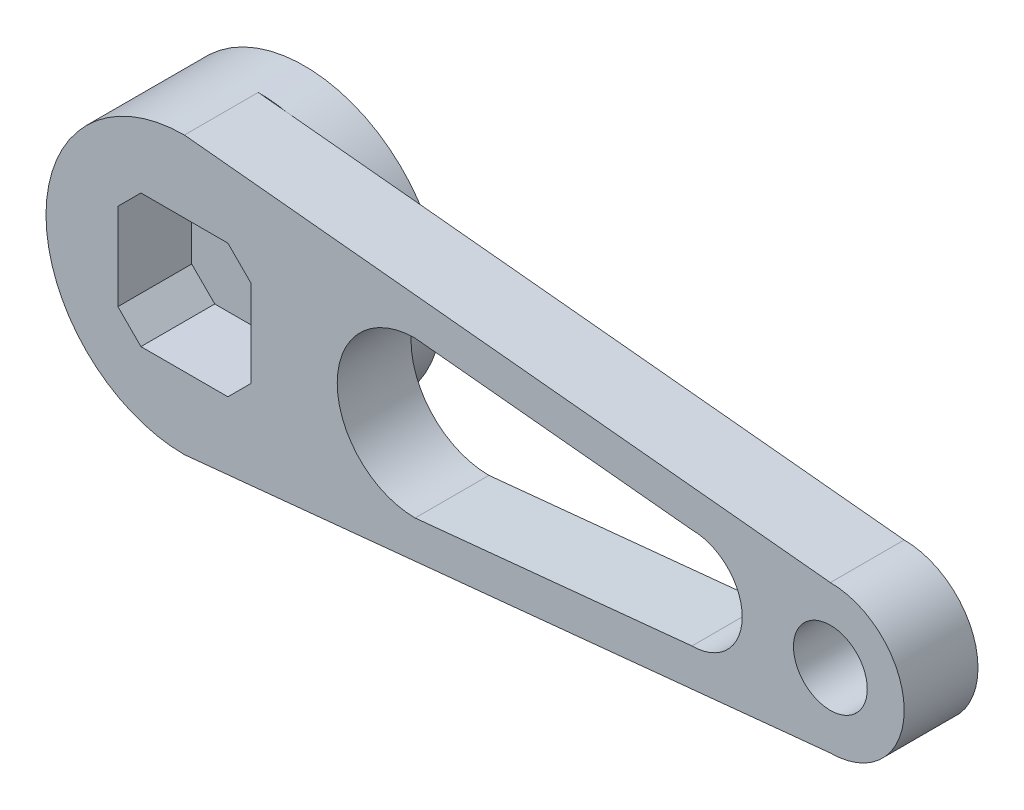
ISO-10303-21;
HEADER;
FILE_DESCRIPTION(('STEP AP214'),'2;1');
FILE_NAME('part.step','',(''),(''),'','','');
FILE_SCHEMA(('AUTOMOTIVE_DESIGN { 1 0 10303 214 1 1 1 1 }'));
ENDSEC;
DATA;
#1=APPLICATION_CONTEXT('core data for automotive mechanical design processes');
#2=APPLICATION_PROTOCOL_DEFINITION('international standard','automotive_design',2000,#1);
#3=PRODUCT_CONTEXT('',#1,'mechanical');
#4=PRODUCT('Part','Part','',(#3));
#5=PRODUCT_RELATED_PRODUCT_CATEGORY('part','',(#4));
#6=PRODUCT_DEFINITION_FORMATION('','',#4);
#7=PRODUCT_DEFINITION_CONTEXT('part definition',#1,'design');
#8=PRODUCT_DEFINITION('design','',#6,#7);
#9=PRODUCT_DEFINITION_SHAPE('','',#8);
#10=(LENGTH_UNIT() NAMED_UNIT(*) SI_UNIT(.MILLI.,.METRE.));
#11=(NAMED_UNIT(*) PLANE_ANGLE_UNIT() SI_UNIT($,.RADIAN.));
#12=(NAMED_UNIT(*) SI_UNIT($,.STERADIAN.) SOLID_ANGLE_UNIT());
#13=UNCERTAINTY_MEASURE_WITH_UNIT(LENGTH_MEASURE(1.E-05),#10,'distance_accuracy_value','');
#14=(GEOMETRIC_REPRESENTATION_CONTEXT(3) GLOBAL_UNCERTAINTY_ASSIGNED_CONTEXT((#13)) GLOBAL_UNIT_ASSIGNED_CONTEXT((#10,
#11,#12)) REPRESENTATION_CONTEXT('',''));
#15=CARTESIAN_POINT('',(0.,0.,0.));
#16=DIRECTION('',(0.,0.,1.));
#17=DIRECTION('',(1.,0.,0.));
#18=AXIS2_PLACEMENT_3D('',#15,#16,#17);
#19=CARTESIAN_POINT('',(0.,0.,0.));
#20=DIRECTION('',(0.,0.,1.));
#21=DIRECTION('',(1.,0.,0.));
#22=AXIS2_PLACEMENT_3D('',#19,#20,#21);
#23=PLANE('',#22);
#24=CARTESIAN_POINT('',(70.,0.,0.));
#25=DIRECTION('',(0.,0.,1.));
#26=DIRECTION('',(1.,0.,0.));
#27=AXIS2_PLACEMENT_3D('',#24,#25,#26);
#28=CIRCLE('',#27,4.00000000000001);
#29=CARTESIAN_POINT('',(74.,0.,0.));
#30=VERTEX_POINT('',#29);
#31=EDGE_CURVE('E238',#30,#30,#28,.T.);
#32=ORIENTED_EDGE('',*,*,#31,.T.);
#33=EDGE_LOOP('',(#32));
#34=FACE_BOUND('',#33,.T.);
#35=DIRECTION('',(-0.995069976609091,0.0991753076687063,0.));
#36=VECTOR('',#35,1.);
#37=CARTESIAN_POINT('',(25.,8.44,0.));
#38=LINE('',#37,#36);
#39=CARTESIAN_POINT('',(55.,5.45,0.));
#40=VERTEX_POINT('',#39);
#41=CARTESIAN_POINT('',(25.,8.44,0.));
#42=VERTEX_POINT('',#41);
#43=EDGE_CURVE('E259',#40,#42,#38,.T.);
#44=ORIENTED_EDGE('',*,*,#43,.T.);
#45=CARTESIAN_POINT('',(25.,0.,0.));
#46=DIRECTION('',(0.,0.,1.));
#47=DIRECTION('',(1.,0.,0.));
#48=AXIS2_PLACEMENT_3D('',#45,#46,#47);
#49=CIRCLE('',#48,8.44);
#50=CARTESIAN_POINT('',(25.,-8.44,0.));
#51=VERTEX_POINT('',#50);
#52=EDGE_CURVE('E246',#42,#51,#49,.T.);
#53=ORIENTED_EDGE('',*,*,#52,.T.);
#54=DIRECTION('',(0.995069976609091,0.0991753076687084,0.));
#55=VECTOR('',#54,1.);
#56=CARTESIAN_POINT('',(25.,-8.44,0.));
#57=LINE('',#56,#55);
#58=CARTESIAN_POINT('',(55.,-5.44999999999994,0.));
#59=VERTEX_POINT('',#58);
#60=EDGE_CURVE('E252',#51,#59,#57,.T.);
#61=ORIENTED_EDGE('',*,*,#60,.T.);
#62=CARTESIAN_POINT('',(55.,0.,0.));
#63=DIRECTION('',(0.,0.,1.));
#64=DIRECTION('',(1.,0.,0.));
#65=AXIS2_PLACEMENT_3D('',#62,#63,#64);
#66=CIRCLE('',#65,5.44999999999997);
#67=EDGE_CURVE('E258',#59,#40,#66,.T.);
#68=ORIENTED_EDGE('',*,*,#67,.T.);
#69=EDGE_LOOP('',(#44,#53,#61,#68));
#70=FACE_BOUND('',#69,.T.);
#71=CARTESIAN_POINT('',(0.,0.,0.));
#72=DIRECTION('',(0.,0.,-1.));
#73=DIRECTION('',(-1.,0.,0.));
#74=AXIS2_PLACEMENT_3D('',#71,#72,#73);
#75=CIRCLE('',#74,15.);
#76=CARTESIAN_POINT('',(2.97029702970299,14.7029702970297,0.));
#77=VERTEX_POINT('',#76);
#78=CARTESIAN_POINT('',(2.97029702970299,-14.7029702970297,0.));
#79=VERTEX_POINT('',#78);
#80=EDGE_CURVE('E11',#77,#79,#75,.T.);
#81=ORIENTED_EDGE('',*,*,#80,.F.);
#82=DIRECTION('',(-0.995037190209989,0.0995037190209989,0.));
#83=VECTOR('',#82,1.);
#84=CARTESIAN_POINT('',(0.,15.,0.));
#85=LINE('',#84,#83);
#86=CARTESIAN_POINT('',(70.,8.,0.));
#87=VERTEX_POINT('',#86);
#88=EDGE_CURVE('E282',#87,#77,#85,.T.);
#89=ORIENTED_EDGE('',*,*,#88,.F.);
#90=CARTESIAN_POINT('',(70.,0.,0.));
#91=DIRECTION('',(0.,0.,1.));
#92=DIRECTION('',(1.,0.,0.));
#93=AXIS2_PLACEMENT_3D('',#90,#91,#92);
#94=CIRCLE('',#93,8.);
#95=CARTESIAN_POINT('',(70.,-8.,0.));
#96=VERTEX_POINT('',#95);
#97=EDGE_CURVE('E294',#96,#87,#94,.T.);
#98=ORIENTED_EDGE('',*,*,#97,.F.);
#99=DIRECTION('',(0.995037190209989,0.0995037190209989,0.));
#100=VECTOR('',#99,1.);
#101=CARTESIAN_POINT('',(0.,-15.,0.));
#102=LINE('',#101,#100);
#103=EDGE_CURVE('E273',#79,#96,#102,.T.);
#104=ORIENTED_EDGE('',*,*,#103,.F.);
#105=EDGE_LOOP('',(#81,#89,#98,#104));
#106=FACE_BOUND('',#105,.T.);
#107=ADVANCED_FACE('F44',(#34,#70,#106),#23,.F.);
#108=CARTESIAN_POINT('',(0.,0.,8.));
#109=DIRECTION('',(0.,0.,-1.));
#110=DIRECTION('',(-1.,0.,0.));
#111=AXIS2_PLACEMENT_3D('',#108,#109,#110);
#112=CYLINDRICAL_SURFACE('',#111,15.);
#113=DIRECTION('',(0.,0.,-1.));
#114=VECTOR('',#113,1.);
#115=CARTESIAN_POINT('',(0.,15.,8.));
#116=LINE('',#115,#114);
#117=CARTESIAN_POINT('',(0.,15.,8.));
#118=VERTEX_POINT('',#117);
#119=CARTESIAN_POINT('',(0.,15.,0.));
#120=VERTEX_POINT('',#119);
#121=EDGE_CURVE('E288',#118,#120,#116,.T.);
#122=ORIENTED_EDGE('',*,*,#121,.T.);
#123=EDGE_CURVE('E54',#120,#77,#75,.T.);
#124=ORIENTED_EDGE('',*,*,#123,.T.);
#125=ORIENTED_EDGE('',*,*,#80,.T.);
#126=CARTESIAN_POINT('',(0.,-15.,0.));
#127=VERTEX_POINT('',#126);
#128=EDGE_CURVE('E57',#79,#127,#75,.T.);
#129=ORIENTED_EDGE('',*,*,#128,.T.);
#130=DIRECTION('',(0.,0.,-1.));
#131=VECTOR('',#130,1.);
#132=CARTESIAN_POINT('',(0.,-15.,8.));
#133=LINE('',#132,#131);
#134=CARTESIAN_POINT('',(0.,-15.,8.));
#135=VERTEX_POINT('',#134);
#136=EDGE_CURVE('E47',#135,#127,#133,.T.);
#137=ORIENTED_EDGE('',*,*,#136,.F.);
#138=CARTESIAN_POINT('',(0.,0.,8.));
#139=DIRECTION('',(0.,0.,1.));
#140=DIRECTION('',(1.,0.,0.));
#141=AXIS2_PLACEMENT_3D('',#138,#139,#140);
#142=CIRCLE('',#141,15.);
#143=EDGE_CURVE('E278',#118,#135,#142,.T.);
#144=ORIENTED_EDGE('',*,*,#143,.F.);
#145=EDGE_LOOP('',(#122,#124,#125,#129,#137,#144));
#146=FACE_BOUND('',#145,.T.);
#147=CARTESIAN_POINT('',(0.,0.,-5.));
#148=DIRECTION('',(0.,0.,-1.));
#149=DIRECTION('',(-1.,0.,0.));
#150=AXIS2_PLACEMENT_3D('',#147,#148,#149);
#151=CIRCLE('',#150,15.);
#152=CARTESIAN_POINT('',(-15.,0.,-5.));
#153=VERTEX_POINT('',#152);
#154=EDGE_CURVE('E244',#153,#153,#151,.T.);
#155=ORIENTED_EDGE('',*,*,#154,.F.);
#156=EDGE_LOOP('',(#155));
#157=FACE_BOUND('',#156,.T.);
#158=ADVANCED_FACE('F50',(#146,#157),#112,.T.);
#159=CARTESIAN_POINT('',(0.,-15.,8.));
#160=DIRECTION('',(-0.0995037190209989,0.995037190209989,0.));
#161=DIRECTION('',(-0.995037190209989,-0.0995037190209989,0.));
#162=AXIS2_PLACEMENT_3D('',#159,#160,#161);
#163=PLANE('',#162);
#164=EDGE_CURVE('E292',#127,#79,#102,.T.);
#165=ORIENTED_EDGE('',*,*,#164,.T.);
#166=ORIENTED_EDGE('',*,*,#103,.T.);
#167=DIRECTION('',(0.,0.,-1.));
#168=VECTOR('',#167,1.);
#169=CARTESIAN_POINT('',(70.,-8.,8.));
#170=LINE('',#169,#168);
#171=CARTESIAN_POINT('',(70.,-8.,8.));
#172=VERTEX_POINT('',#171);
#173=EDGE_CURVE('E305',#172,#96,#170,.T.);
#174=ORIENTED_EDGE('',*,*,#173,.F.);
#175=DIRECTION('',(0.995037190209989,0.0995037190209989,0.));
#176=VECTOR('',#175,1.);
#177=CARTESIAN_POINT('',(0.,-15.,8.));
#178=LINE('',#177,#176);
#179=EDGE_CURVE('E281',#135,#172,#178,.T.);
#180=ORIENTED_EDGE('',*,*,#179,.F.);
#181=ORIENTED_EDGE('',*,*,#136,.T.);
#182=EDGE_LOOP('',(#165,#166,#174,#180,#181));
#183=FACE_BOUND('',#182,.T.);
#184=ADVANCED_FACE('F315',(#183),#163,.F.);
#185=CARTESIAN_POINT('',(70.,0.,8.));
#186=DIRECTION('',(0.,0.,-1.));
#187=DIRECTION('',(-1.,0.,0.));
#188=AXIS2_PLACEMENT_3D('',#185,#186,#187);
#189=CYLINDRICAL_SURFACE('',#188,8.);
#190=ORIENTED_EDGE('',*,*,#97,.T.);
#191=DIRECTION('',(0.,0.,-1.));
#192=VECTOR('',#191,1.);
#193=CARTESIAN_POINT('',(70.,8.,8.));
#194=LINE('',#193,#192);
#195=CARTESIAN_POINT('',(70.,8.,8.));
#196=VERTEX_POINT('',#195);
#197=EDGE_CURVE('E302',#196,#87,#194,.T.);
#198=ORIENTED_EDGE('',*,*,#197,.F.);
#199=CARTESIAN_POINT('',(70.,0.,8.));
#200=DIRECTION('',(0.,0.,1.));
#201=DIRECTION('',(1.,0.,0.));
#202=AXIS2_PLACEMENT_3D('',#199,#200,#201);
#203=CIRCLE('',#202,8.);
#204=EDGE_CURVE('E287',#172,#196,#203,.T.);
#205=ORIENTED_EDGE('',*,*,#204,.F.);
#206=ORIENTED_EDGE('',*,*,#173,.T.);
#207=EDGE_LOOP('',(#190,#198,#205,#206));
#208=FACE_BOUND('',#207,.T.);
#209=ADVANCED_FACE('F354',(#208),#189,.T.);
#210=CARTESIAN_POINT('',(0.,15.,8.));
#211=DIRECTION('',(-0.0995037190209989,-0.995037190209989,0.));
#212=DIRECTION('',(0.995037190209989,-0.0995037190209989,0.));
#213=AXIS2_PLACEMENT_3D('',#210,#211,#212);
#214=PLANE('',#213);
#215=ORIENTED_EDGE('',*,*,#88,.T.);
#216=EDGE_CURVE('E298',#77,#120,#85,.T.);
#217=ORIENTED_EDGE('',*,*,#216,.T.);
#218=ORIENTED_EDGE('',*,*,#121,.F.);
#219=DIRECTION('',(-0.995037190209989,0.0995037190209989,0.));
#220=VECTOR('',#219,1.);
#221=CARTESIAN_POINT('',(0.,15.,8.));
#222=LINE('',#221,#220);
#223=EDGE_CURVE('E290',#196,#118,#222,.T.);
#224=ORIENTED_EDGE('',*,*,#223,.F.);
#225=ORIENTED_EDGE('',*,*,#197,.T.);
#226=EDGE_LOOP('',(#215,#217,#218,#224,#225));
#227=FACE_BOUND('',#226,.T.);
#228=ADVANCED_FACE('F355',(#227),#214,.F.);
#229=CARTESIAN_POINT('',(0.,0.,8.));
#230=DIRECTION('',(0.,0.,1.));
#231=DIRECTION('',(1.,0.,0.));
#232=AXIS2_PLACEMENT_3D('',#229,#230,#231);
#233=PLANE('',#232);
#234=DIRECTION('',(-0.707106781186548,0.707106781186547,0.));
#235=VECTOR('',#234,1.);
#236=CARTESIAN_POINT('',(7.21,4.71,8.));
#237=LINE('',#236,#235);
#238=CARTESIAN_POINT('',(7.21,4.71,8.));
#239=VERTEX_POINT('',#238);
#240=CARTESIAN_POINT('',(4.71,7.21,8.));
#241=VERTEX_POINT('',#240);
#242=EDGE_CURVE('E61',#239,#241,#237,.T.);
#243=ORIENTED_EDGE('',*,*,#242,.F.);
#244=DIRECTION('',(0.,1.,0.));
#245=VECTOR('',#244,1.);
#246=CARTESIAN_POINT('',(7.21,-4.71000000000001,8.));
#247=LINE('',#246,#245);
#248=CARTESIAN_POINT('',(7.21,-4.71000000000001,8.));
#249=VERTEX_POINT('',#248);
#250=EDGE_CURVE('E225',#249,#239,#247,.T.);
#251=ORIENTED_EDGE('',*,*,#250,.F.);
#252=DIRECTION('',(0.707106781186549,0.707106781186546,0.));
#253=VECTOR('',#252,1.);
#254=CARTESIAN_POINT('',(4.71,-7.21,8.));
#255=LINE('',#254,#253);
#256=CARTESIAN_POINT('',(4.71,-7.21,8.));
#257=VERTEX_POINT('',#256);
#258=EDGE_CURVE('E218',#257,#249,#255,.T.);
#259=ORIENTED_EDGE('',*,*,#258,.F.);
#260=DIRECTION('',(1.,0.,0.));
#261=VECTOR('',#260,1.);
#262=CARTESIAN_POINT('',(-4.71,-7.21,8.));
#263=LINE('',#262,#261);
#264=CARTESIAN_POINT('',(-4.71,-7.21,8.));
#265=VERTEX_POINT('',#264);
#266=EDGE_CURVE('E216',#265,#257,#263,.T.);
#267=ORIENTED_EDGE('',*,*,#266,.F.);
#268=DIRECTION('',(0.707106781186549,-0.707106781186546,0.));
#269=VECTOR('',#268,1.);
#270=CARTESIAN_POINT('',(-4.71,-7.21,8.));
#271=LINE('',#270,#269);
#272=CARTESIAN_POINT('',(-7.21,-4.71000000000001,8.));
#273=VERTEX_POINT('',#272);
#274=EDGE_CURVE('E213',#273,#265,#271,.T.);
#275=ORIENTED_EDGE('',*,*,#274,.F.);
#276=DIRECTION('',(0.,-1.,0.));
#277=VECTOR('',#276,1.);
#278=CARTESIAN_POINT('',(-7.21,4.71,8.));
#279=LINE('',#278,#277);
#280=CARTESIAN_POINT('',(-7.21,4.71,8.));
#281=VERTEX_POINT('',#280);
#282=EDGE_CURVE('E209',#281,#273,#279,.T.);
#283=ORIENTED_EDGE('',*,*,#282,.F.);
#284=DIRECTION('',(-0.707106781186548,-0.707106781186547,0.));
#285=VECTOR('',#284,1.);
#286=CARTESIAN_POINT('',(-7.21,4.71,8.));
#287=LINE('',#286,#285);
#288=CARTESIAN_POINT('',(-4.71,7.21,8.));
#289=VERTEX_POINT('',#288);
#290=EDGE_CURVE('E208',#289,#281,#287,.T.);
#291=ORIENTED_EDGE('',*,*,#290,.F.);
#292=DIRECTION('',(-1.,0.,0.));
#293=VECTOR('',#292,1.);
#294=CARTESIAN_POINT('',(0.,7.21,8.));
#295=LINE('',#294,#293);
#296=EDGE_CURVE('E181',#241,#289,#295,.T.);
#297=ORIENTED_EDGE('',*,*,#296,.F.);
#298=EDGE_LOOP('',(#243,#251,#259,#267,#275,#283,#291,#297));
#299=FACE_BOUND('',#298,.T.);
#300=CARTESIAN_POINT('',(70.,0.,8.));
#301=DIRECTION('',(0.,0.,1.));
#302=DIRECTION('',(1.,0.,0.));
#303=AXIS2_PLACEMENT_3D('',#300,#301,#302);
#304=CIRCLE('',#303,4.00000000000001);
#305=CARTESIAN_POINT('',(74.,0.,8.));
#306=VERTEX_POINT('',#305);
#307=EDGE_CURVE('E226',#306,#306,#304,.T.);
#308=ORIENTED_EDGE('',*,*,#307,.F.);
#309=EDGE_LOOP('',(#308));
#310=FACE_BOUND('',#309,.T.);
#311=CARTESIAN_POINT('',(25.,0.,8.));
#312=DIRECTION('',(0.,0.,1.));
#313=DIRECTION('',(1.,0.,0.));
#314=AXIS2_PLACEMENT_3D('',#311,#312,#313);
#315=CIRCLE('',#314,8.44);
#316=CARTESIAN_POINT('',(25.,8.44,8.));
#317=VERTEX_POINT('',#316);
#318=CARTESIAN_POINT('',(25.,-8.44,8.));
#319=VERTEX_POINT('',#318);
#320=EDGE_CURVE('E72',#317,#319,#315,.T.);
#321=ORIENTED_EDGE('',*,*,#320,.F.);
#322=DIRECTION('',(-0.995069976609091,0.0991753076687063,0.));
#323=VECTOR('',#322,1.);
#324=CARTESIAN_POINT('',(25.,8.44,8.));
#325=LINE('',#324,#323);
#326=CARTESIAN_POINT('',(55.,5.45,8.));
#327=VERTEX_POINT('',#326);
#328=EDGE_CURVE('E251',#327,#317,#325,.T.);
#329=ORIENTED_EDGE('',*,*,#328,.F.);
#330=CARTESIAN_POINT('',(55.,0.,8.));
#331=DIRECTION('',(0.,0.,1.));
#332=DIRECTION('',(1.,0.,0.));
#333=AXIS2_PLACEMENT_3D('',#330,#331,#332);
#334=CIRCLE('',#333,5.44999999999997);
#335=CARTESIAN_POINT('',(55.,-5.44999999999997,8.));
#336=VERTEX_POINT('',#335);
#337=EDGE_CURVE('E270',#336,#327,#334,.T.);
#338=ORIENTED_EDGE('',*,*,#337,.F.);
#339=DIRECTION('',(0.995069976609091,0.0991753076687084,0.));
#340=VECTOR('',#339,1.);
#341=CARTESIAN_POINT('',(25.,-8.44,8.));
#342=LINE('',#341,#340);
#343=EDGE_CURVE('E262',#319,#336,#342,.T.);
#344=ORIENTED_EDGE('',*,*,#343,.F.);
#345=EDGE_LOOP('',(#321,#329,#338,#344));
#346=FACE_BOUND('',#345,.T.);
#347=ORIENTED_EDGE('',*,*,#143,.T.);
#348=ORIENTED_EDGE('',*,*,#179,.T.);
#349=ORIENTED_EDGE('',*,*,#204,.T.);
#350=ORIENTED_EDGE('',*,*,#223,.T.);
#351=EDGE_LOOP('',(#347,#348,#349,#350));
#352=FACE_BOUND('',#351,.T.);
#353=ADVANCED_FACE('F348',(#299,#310,#346,#352),#233,.T.);
#354=CARTESIAN_POINT('',(25.,0.,0.));
#355=DIRECTION('',(0.,0.,1.));
#356=DIRECTION('',(1.,0.,0.));
#357=AXIS2_PLACEMENT_3D('',#354,#355,#356);
#358=CYLINDRICAL_SURFACE('',#357,8.44);
#359=ORIENTED_EDGE('',*,*,#320,.T.);
#360=DIRECTION('',(0.,0.,1.));
#361=VECTOR('',#360,1.);
#362=CARTESIAN_POINT('',(25.,-8.44,0.));
#363=LINE('',#362,#361);
#364=EDGE_CURVE('E265',#51,#319,#363,.T.);
#365=ORIENTED_EDGE('',*,*,#364,.F.);
#366=ORIENTED_EDGE('',*,*,#52,.F.);
#367=DIRECTION('',(0.,0.,1.));
#368=VECTOR('',#367,1.);
#369=CARTESIAN_POINT('',(25.,8.44,0.));
#370=LINE('',#369,#368);
#371=EDGE_CURVE('E275',#42,#317,#370,.T.);
#372=ORIENTED_EDGE('',*,*,#371,.T.);
#373=EDGE_LOOP('',(#359,#365,#366,#372));
#374=FACE_BOUND('',#373,.T.);
#375=ADVANCED_FACE('F425',(#374),#358,.F.);
#376=CARTESIAN_POINT('',(25.,8.44,0.));
#377=DIRECTION('',(0.0991753076687063,0.995069976609091,0.));
#378=DIRECTION('',(-0.995069976609091,0.0991753076687063,0.));
#379=AXIS2_PLACEMENT_3D('',#376,#377,#378);
#380=PLANE('',#379);
#381=ORIENTED_EDGE('',*,*,#328,.T.);
#382=ORIENTED_EDGE('',*,*,#371,.F.);
#383=ORIENTED_EDGE('',*,*,#43,.F.);
#384=DIRECTION('',(0.,0.,1.));
#385=VECTOR('',#384,1.);
#386=CARTESIAN_POINT('',(55.,5.45,0.));
#387=LINE('',#386,#385);
#388=EDGE_CURVE('E274',#40,#327,#387,.T.);
#389=ORIENTED_EDGE('',*,*,#388,.T.);
#390=EDGE_LOOP('',(#381,#382,#383,#389));
#391=FACE_BOUND('',#390,.T.);
#392=ADVANCED_FACE('F422',(#391),#380,.F.);
#393=CARTESIAN_POINT('',(55.,0.,0.));
#394=DIRECTION('',(0.,0.,1.));
#395=DIRECTION('',(1.,0.,0.));
#396=AXIS2_PLACEMENT_3D('',#393,#394,#395);
#397=CYLINDRICAL_SURFACE('',#396,5.44999999999997);
#398=ORIENTED_EDGE('',*,*,#337,.T.);
#399=ORIENTED_EDGE('',*,*,#388,.F.);
#400=ORIENTED_EDGE('',*,*,#67,.F.);
#401=DIRECTION('',(0.,0.,1.));
#402=VECTOR('',#401,1.);
#403=CARTESIAN_POINT('',(55.,-5.44999999999997,0.));
#404=LINE('',#403,#402);
#405=EDGE_CURVE('E280',#59,#336,#404,.T.);
#406=ORIENTED_EDGE('',*,*,#405,.T.);
#407=EDGE_LOOP('',(#398,#399,#400,#406));
#408=FACE_BOUND('',#407,.T.);
#409=ADVANCED_FACE('F433',(#408),#397,.F.);
#410=CARTESIAN_POINT('',(25.,-8.44,0.));
#411=DIRECTION('',(0.0991753076687084,-0.995069976609091,0.));
#412=DIRECTION('',(0.995069976609091,0.0991753076687084,0.));
#413=AXIS2_PLACEMENT_3D('',#410,#411,#412);
#414=PLANE('',#413);
#415=ORIENTED_EDGE('',*,*,#343,.T.);
#416=ORIENTED_EDGE('',*,*,#405,.F.);
#417=ORIENTED_EDGE('',*,*,#60,.F.);
#418=ORIENTED_EDGE('',*,*,#364,.T.);
#419=EDGE_LOOP('',(#415,#416,#417,#418));
#420=FACE_BOUND('',#419,.T.);
#421=ADVANCED_FACE('F337',(#420),#414,.F.);
#422=CARTESIAN_POINT('',(0.,0.,0.));
#423=DIRECTION('',(0.,0.,-1.));
#424=DIRECTION('',(-1.,0.,0.));
#425=AXIS2_PLACEMENT_3D('',#422,#423,#424);
#426=PLANE('',#425);
#427=ORIENTED_EDGE('',*,*,#216,.F.);
#428=ORIENTED_EDGE('',*,*,#123,.F.);
#429=EDGE_LOOP('',(#427,#428));
#430=FACE_BOUND('',#429,.T.);
#431=ADVANCED_FACE('F324',(#430),#426,.F.);
#432=CARTESIAN_POINT('',(0.,0.,-5.));
#433=DIRECTION('',(0.,0.,-1.));
#434=DIRECTION('',(-1.,0.,0.));
#435=AXIS2_PLACEMENT_3D('',#432,#433,#434);
#436=PLANE('',#435);
#437=ORIENTED_EDGE('',*,*,#154,.T.);
#438=EDGE_LOOP('',(#437));
#439=FACE_BOUND('',#438,.T.);
#440=ADVANCED_FACE('F323',(#439),#436,.T.);
#441=ORIENTED_EDGE('',*,*,#164,.F.);
#442=ORIENTED_EDGE('',*,*,#128,.F.);
#443=EDGE_LOOP('',(#441,#442));
#444=FACE_BOUND('',#443,.T.);
#445=ADVANCED_FACE('F319',(#444),#426,.F.);
#446=CARTESIAN_POINT('',(70.,0.,0.));
#447=DIRECTION('',(0.,0.,1.));
#448=DIRECTION('',(1.,0.,0.));
#449=AXIS2_PLACEMENT_3D('',#446,#447,#448);
#450=CYLINDRICAL_SURFACE('',#449,4.00000000000001);
#451=ORIENTED_EDGE('',*,*,#31,.F.);
#452=EDGE_LOOP('',(#451));
#453=FACE_BOUND('',#452,.T.);
#454=ORIENTED_EDGE('',*,*,#307,.T.);
#455=EDGE_LOOP('',(#454));
#456=FACE_BOUND('',#455,.T.);
#457=ADVANCED_FACE('F325',(#453,#456),#450,.F.);
#458=CARTESIAN_POINT('',(7.21,4.71,0.));
#459=DIRECTION('',(0.707106781186547,0.707106781186548,0.));
#460=DIRECTION('',(-0.707106781186548,0.707106781186547,0.));
#461=AXIS2_PLACEMENT_3D('',#458,#459,#460);
#462=PLANE('',#461);
#463=ORIENTED_EDGE('',*,*,#242,.T.);
#464=DIRECTION('',(0.,0.,1.));
#465=VECTOR('',#464,1.);
#466=CARTESIAN_POINT('',(4.71,7.21,0.));
#467=LINE('',#466,#465);
#468=CARTESIAN_POINT('',(4.71,7.21,0.));
#469=VERTEX_POINT('',#468);
#470=EDGE_CURVE('E228',#469,#241,#467,.T.);
#471=ORIENTED_EDGE('',*,*,#470,.F.);
#472=DIRECTION('',(-0.707106781186548,0.707106781186547,0.));
#473=VECTOR('',#472,1.);
#474=CARTESIAN_POINT('',(7.21,4.71,0.));
#475=LINE('',#474,#473);
#476=CARTESIAN_POINT('',(7.21,4.71,0.));
#477=VERTEX_POINT('',#476);
#478=EDGE_CURVE('E177',#477,#469,#475,.T.);
#479=ORIENTED_EDGE('',*,*,#478,.F.);
#480=DIRECTION('',(0.,0.,1.));
#481=VECTOR('',#480,1.);
#482=CARTESIAN_POINT('',(7.21,4.71,0.));
#483=LINE('',#482,#481);
#484=EDGE_CURVE('E227',#477,#239,#483,.T.);
#485=ORIENTED_EDGE('',*,*,#484,.T.);
#486=EDGE_LOOP('',(#463,#471,#479,#485));
#487=FACE_BOUND('',#486,.T.);
#488=ADVANCED_FACE('F332',(#487),#462,.F.);
#489=CARTESIAN_POINT('',(7.21,-4.71000000000001,0.));
#490=DIRECTION('',(1.,0.,0.));
#491=DIRECTION('',(0.,0.,-1.));
#492=AXIS2_PLACEMENT_3D('',#489,#490,#491);
#493=PLANE('',#492);
#494=ORIENTED_EDGE('',*,*,#250,.T.);
#495=ORIENTED_EDGE('',*,*,#484,.F.);
#496=DIRECTION('',(0.,1.,0.));
#497=VECTOR('',#496,1.);
#498=CARTESIAN_POINT('',(7.21,-4.71000000000001,0.));
#499=LINE('',#498,#497);
#500=CARTESIAN_POINT('',(7.21,-4.71000000000001,0.));
#501=VERTEX_POINT('',#500);
#502=EDGE_CURVE('E204',#501,#477,#499,.T.);
#503=ORIENTED_EDGE('',*,*,#502,.F.);
#504=DIRECTION('',(0.,0.,1.));
#505=VECTOR('',#504,1.);
#506=CARTESIAN_POINT('',(7.21,-4.71000000000001,0.));
#507=LINE('',#506,#505);
#508=EDGE_CURVE('E232',#501,#249,#507,.T.);
#509=ORIENTED_EDGE('',*,*,#508,.T.);
#510=EDGE_LOOP('',(#494,#495,#503,#509));
#511=FACE_BOUND('',#510,.T.);
#512=ADVANCED_FACE('F458',(#511),#493,.F.);
#513=CARTESIAN_POINT('',(4.71,-7.21,0.));
#514=DIRECTION('',(0.707106781186546,-0.707106781186549,0.));
#515=DIRECTION('',(0.707106781186549,0.707106781186546,0.));
#516=AXIS2_PLACEMENT_3D('',#513,#514,#515);
#517=PLANE('',#516);
#518=ORIENTED_EDGE('',*,*,#258,.T.);
#519=ORIENTED_EDGE('',*,*,#508,.F.);
#520=DIRECTION('',(0.707106781186549,0.707106781186546,0.));
#521=VECTOR('',#520,1.);
#522=CARTESIAN_POINT('',(4.71,-7.21,0.));
#523=LINE('',#522,#521);
#524=CARTESIAN_POINT('',(4.71,-7.21,0.));
#525=VERTEX_POINT('',#524);
#526=EDGE_CURVE('E203',#525,#501,#523,.T.);
#527=ORIENTED_EDGE('',*,*,#526,.F.);
#528=DIRECTION('',(0.,0.,1.));
#529=VECTOR('',#528,1.);
#530=CARTESIAN_POINT('',(4.71,-7.21,0.));
#531=LINE('',#530,#529);
#532=EDGE_CURVE('E235',#525,#257,#531,.T.);
#533=ORIENTED_EDGE('',*,*,#532,.T.);
#534=EDGE_LOOP('',(#518,#519,#527,#533));
#535=FACE_BOUND('',#534,.T.);
#536=ADVANCED_FACE('F469',(#535),#517,.F.);
#537=CARTESIAN_POINT('',(-4.71,-7.21,0.));
#538=DIRECTION('',(0.,-1.,0.));
#539=DIRECTION('',(0.,0.,-1.));
#540=AXIS2_PLACEMENT_3D('',#537,#538,#539);
#541=PLANE('',#540);
#542=ORIENTED_EDGE('',*,*,#266,.T.);
#543=ORIENTED_EDGE('',*,*,#532,.F.);
#544=DIRECTION('',(1.,0.,0.));
#545=VECTOR('',#544,1.);
#546=CARTESIAN_POINT('',(-4.71,-7.21,0.));
#547=LINE('',#546,#545);
#548=CARTESIAN_POINT('',(-4.71,-7.21,0.));
#549=VERTEX_POINT('',#548);
#550=EDGE_CURVE('E196',#549,#525,#547,.T.);
#551=ORIENTED_EDGE('',*,*,#550,.F.);
#552=DIRECTION('',(0.,0.,1.));
#553=VECTOR('',#552,1.);
#554=CARTESIAN_POINT('',(-4.71,-7.21,0.));
#555=LINE('',#554,#553);
#556=EDGE_CURVE('E233',#549,#265,#555,.T.);
#557=ORIENTED_EDGE('',*,*,#556,.T.);
#558=EDGE_LOOP('',(#542,#543,#551,#557));
#559=FACE_BOUND('',#558,.T.);
#560=ADVANCED_FACE('F474',(#559),#541,.F.);
#561=CARTESIAN_POINT('',(-4.71,-7.21,0.));
#562=DIRECTION('',(-0.707106781186546,-0.707106781186549,0.));
#563=DIRECTION('',(0.707106781186549,-0.707106781186546,0.));
#564=AXIS2_PLACEMENT_3D('',#561,#562,#563);
#565=PLANE('',#564);
#566=ORIENTED_EDGE('',*,*,#274,.T.);
#567=ORIENTED_EDGE('',*,*,#556,.F.);
#568=DIRECTION('',(0.707106781186549,-0.707106781186546,0.));
#569=VECTOR('',#568,1.);
#570=CARTESIAN_POINT('',(-4.71,-7.21,0.));
#571=LINE('',#570,#569);
#572=CARTESIAN_POINT('',(-7.21,-4.71000000000001,0.));
#573=VERTEX_POINT('',#572);
#574=EDGE_CURVE('E195',#573,#549,#571,.T.);
#575=ORIENTED_EDGE('',*,*,#574,.F.);
#576=DIRECTION('',(0.,0.,1.));
#577=VECTOR('',#576,1.);
#578=CARTESIAN_POINT('',(-7.21,-4.71000000000001,0.));
#579=LINE('',#578,#577);
#580=EDGE_CURVE('E240',#573,#273,#579,.T.);
#581=ORIENTED_EDGE('',*,*,#580,.T.);
#582=EDGE_LOOP('',(#566,#567,#575,#581));
#583=FACE_BOUND('',#582,.T.);
#584=ADVANCED_FACE('F483',(#583),#565,.F.);
#585=CARTESIAN_POINT('',(-7.21,4.71,0.));
#586=DIRECTION('',(-1.,0.,0.));
#587=DIRECTION('',(0.,0.,1.));
#588=AXIS2_PLACEMENT_3D('',#585,#586,#587);
#589=PLANE('',#588);
#590=ORIENTED_EDGE('',*,*,#282,.T.);
#591=ORIENTED_EDGE('',*,*,#580,.F.);
#592=DIRECTION('',(0.,-1.,0.));
#593=VECTOR('',#592,1.);
#594=CARTESIAN_POINT('',(-7.21,4.71,0.));
#595=LINE('',#594,#593);
#596=CARTESIAN_POINT('',(-7.21,4.71,0.));
#597=VERTEX_POINT('',#596);
#598=EDGE_CURVE('E192',#597,#573,#595,.T.);
#599=ORIENTED_EDGE('',*,*,#598,.F.);
#600=DIRECTION('',(0.,0.,1.));
#601=VECTOR('',#600,1.);
#602=CARTESIAN_POINT('',(-7.21,4.71,0.));
#603=LINE('',#602,#601);
#604=EDGE_CURVE('E190',#597,#281,#603,.T.);
#605=ORIENTED_EDGE('',*,*,#604,.T.);
#606=EDGE_LOOP('',(#590,#591,#599,#605));
#607=FACE_BOUND('',#606,.T.);
#608=ADVANCED_FACE('F491',(#607),#589,.F.);
#609=CARTESIAN_POINT('',(-7.21,4.71,0.));
#610=DIRECTION('',(-0.707106781186547,0.707106781186548,0.));
#611=DIRECTION('',(-0.707106781186548,-0.707106781186547,0.));
#612=AXIS2_PLACEMENT_3D('',#609,#610,#611);
#613=PLANE('',#612);
#614=ORIENTED_EDGE('',*,*,#290,.T.);
#615=ORIENTED_EDGE('',*,*,#604,.F.);
#616=DIRECTION('',(-0.707106781186548,-0.707106781186547,0.));
#617=VECTOR('',#616,1.);
#618=CARTESIAN_POINT('',(-7.21,4.71,0.));
#619=LINE('',#618,#617);
#620=CARTESIAN_POINT('',(-4.71,7.21,0.));
#621=VERTEX_POINT('',#620);
#622=EDGE_CURVE('E171',#621,#597,#619,.T.);
#623=ORIENTED_EDGE('',*,*,#622,.F.);
#624=DIRECTION('',(0.,0.,1.));
#625=VECTOR('',#624,1.);
#626=CARTESIAN_POINT('',(-4.71,7.21,0.));
#627=LINE('',#626,#625);
#628=EDGE_CURVE('E178',#621,#289,#627,.T.);
#629=ORIENTED_EDGE('',*,*,#628,.T.);
#630=EDGE_LOOP('',(#614,#615,#623,#629));
#631=FACE_BOUND('',#630,.T.);
#632=ADVANCED_FACE('F187',(#631),#613,.F.);
#633=CARTESIAN_POINT('',(0.,7.21,0.));
#634=DIRECTION('',(0.,1.,0.));
#635=DIRECTION('',(0.,0.,1.));
#636=AXIS2_PLACEMENT_3D('',#633,#634,#635);
#637=PLANE('',#636);
#638=ORIENTED_EDGE('',*,*,#296,.T.);
#639=ORIENTED_EDGE('',*,*,#628,.F.);
#640=DIRECTION('',(-1.,0.,0.));
#641=VECTOR('',#640,1.);
#642=CARTESIAN_POINT('',(4.71,7.21,0.));
#643=LINE('',#642,#641);
#644=EDGE_CURVE('E169',#469,#621,#643,.T.);
#645=ORIENTED_EDGE('',*,*,#644,.F.);
#646=ORIENTED_EDGE('',*,*,#470,.T.);
#647=EDGE_LOOP('',(#638,#639,#645,#646));
#648=FACE_BOUND('',#647,.T.);
#649=ADVANCED_FACE('F182',(#648),#637,.F.);
#650=CARTESIAN_POINT('',(0.,0.,0.));
#651=DIRECTION('',(0.,0.,1.));
#652=DIRECTION('',(1.,0.,0.));
#653=AXIS2_PLACEMENT_3D('',#650,#651,#652);
#654=PLANE('',#653);
#655=ORIENTED_EDGE('',*,*,#644,.T.);
#656=ORIENTED_EDGE('',*,*,#622,.T.);
#657=ORIENTED_EDGE('',*,*,#598,.T.);
#658=ORIENTED_EDGE('',*,*,#574,.T.);
#659=ORIENTED_EDGE('',*,*,#550,.T.);
#660=ORIENTED_EDGE('',*,*,#526,.T.);
#661=ORIENTED_EDGE('',*,*,#502,.T.);
#662=ORIENTED_EDGE('',*,*,#478,.T.);
#663=EDGE_LOOP('',(#655,#656,#657,#658,#659,#660,#661,#662));
#664=FACE_BOUND('',#663,.T.);
#665=ADVANCED_FACE('F168',(#664),#654,.T.);
#666=CLOSED_SHELL('',(#107,#158,#184,#209,#228,#353,#375,#392,#409,#421,#431,#440,#445,#457,
#488,#512,#536,#560,#584,#608,#632,#649,#665));
#667=MANIFOLD_SOLID_BREP('B2',#666);
#668=ADVANCED_BREP_SHAPE_REPRESENTATION('',(#18,#667),#14);
#669=SHAPE_DEFINITION_REPRESENTATION(#9,#668);
ENDSEC;
END-ISO-10303-21;
